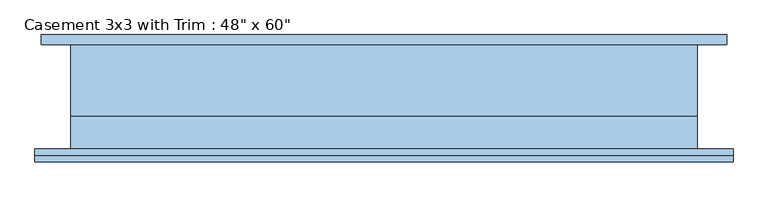
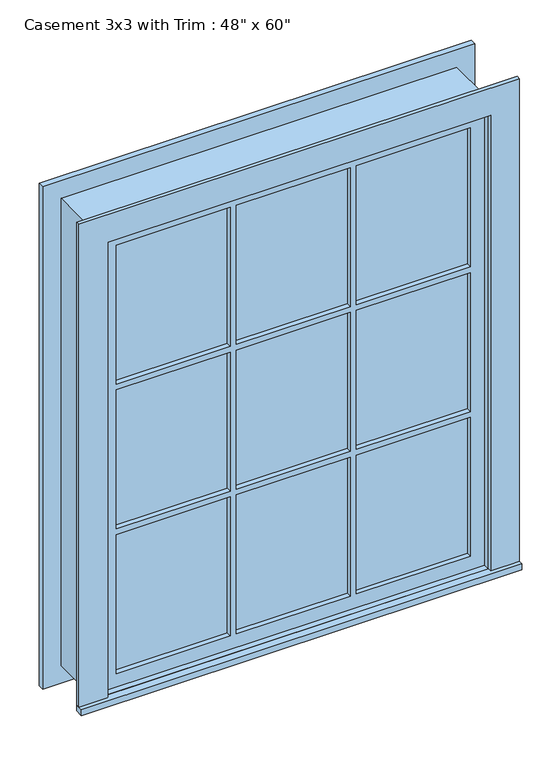
"""IFC4 building model written with IfcOpenShell, lengths in millimetres: window geometry."""

from ifc_helpers import new_model, si_unit, frame, origin, place, context, project, spatial, polyline, outline, extrude, source, transform, mapped, element, save


def window_4f803b43(model_context):
    return source(origin(), model_context, "Body", "SweptSolid", [
        extrude(outline(polyline([(-679.45, -127.0), (-679.45, -101.6), (679.45, -101.6), (679.45, -127.0), (-679.45, -127.0)])), frame((0.0, 0.0, 609.6), z_axis=(0.0, 0.0, 1.0), x_axis=(1.0, 0.0, 0.0)), (0.0, 0.0, 1.0), 19.05),
        extrude(outline(polyline([(2114.55, -590.55), (2114.55, 590.55), (628.65, 590.55), (628.65, 679.45), (2203.45, 679.45), (2203.45, -679.45), (628.65, -679.45), (628.65, -590.55), (2114.55, -590.55)])), frame((0.0, -114.3, 0.0), z_axis=(0.0, 1.0, 0.0), x_axis=(0.0, 0.0, 1.0)), (0.0, 0.0, 1.0), 12.7),
        extrude(outline(polyline([(194.7333333, -66.675), (194.7333333, -53.975), (546.1, -53.975), (546.1, -66.675), (194.7333333, -66.675)])), frame((0.0, 0.0, 1617.1333333), z_axis=(0.0, 0.0, 1.0), x_axis=(1.0, 0.0, 0.0)), (0.0, 0.0, 1.0), 452.9666667),
        extrude(outline(polyline([(-175.6833333, -66.675), (-175.6833333, -53.975), (175.6833333, -53.975), (175.6833333, -66.675), (-175.6833333, -66.675)])), frame((0.0, 0.0, 1617.1333333), z_axis=(0.0, 0.0, 1.0), x_axis=(1.0, 0.0, 0.0)), (0.0, 0.0, 1.0), 452.9666667),
        extrude(outline(polyline([(-546.1, -66.675), (-546.1, -53.975), (-194.7333333, -53.975), (-194.7333333, -66.675), (-546.1, -66.675)])), frame((0.0, 0.0, 1617.1333333), z_axis=(0.0, 0.0, 1.0), x_axis=(1.0, 0.0, 0.0)), (0.0, 0.0, 1.0), 452.9666667),
        extrude(outline(polyline([(-546.1, -66.675), (-546.1, -53.975), (-194.7333333, -53.975), (-194.7333333, -66.675), (-546.1, -66.675)])), frame((0.0, 0.0, 1145.1166667), z_axis=(0.0, 0.0, 1.0), x_axis=(1.0, 0.0, 0.0)), (0.0, 0.0, 1.0), 452.9666667),
        extrude(outline(polyline([(-175.6833333, -66.675), (-175.6833333, -53.975), (175.6833333, -53.975), (175.6833333, -66.675), (-175.6833333, -66.675)])), frame((0.0, 0.0, 1145.1166667), z_axis=(0.0, 0.0, 1.0), x_axis=(1.0, 0.0, 0.0)), (0.0, 0.0, 1.0), 452.9666667),
        extrude(outline(polyline([(194.7333333, -66.675), (194.7333333, -53.975), (546.1, -53.975), (546.1, -66.675), (194.7333333, -66.675)])), frame((0.0, 0.0, 1145.1166667), z_axis=(0.0, 0.0, 1.0), x_axis=(1.0, 0.0, 0.0)), (0.0, 0.0, 1.0), 452.9666667),
        extrude(outline(polyline([(194.7333333, -66.675), (194.7333333, -53.975), (546.1, -53.975), (546.1, -66.675), (194.7333333, -66.675)])), frame((0.0, 0.0, 673.1), z_axis=(0.0, 0.0, 1.0), x_axis=(1.0, 0.0, 0.0)), (0.0, 0.0, 1.0), 452.9666667),
        extrude(outline(polyline([(-175.6833333, -66.675), (-175.6833333, -53.975), (175.6833333, -53.975), (175.6833333, -66.675), (-175.6833333, -66.675)])), frame((0.0, 0.0, 673.1), z_axis=(0.0, 0.0, 1.0), x_axis=(1.0, 0.0, 0.0)), (0.0, 0.0, 1.0), 452.9666667),
        extrude(outline(polyline([(-546.1, -66.675), (-546.1, -53.975), (-194.7333333, -53.975), (-194.7333333, -66.675), (-546.1, -66.675)])), frame((0.0, 0.0, 673.1), z_axis=(0.0, 0.0, 1.0), x_axis=(1.0, 0.0, 0.0)), (0.0, 0.0, 1.0), 452.9666667),
        extrude(outline(polyline([(2190.75, 666.75), (2190.75, -666.75), (552.45, -666.75), (552.45, 666.75), (2190.75, 666.75)]), holes=[polyline([(2101.85, 577.85), (641.35, 577.85), (641.35, -577.85), (2101.85, -577.85), (2101.85, 577.85)])]), frame((0.0, 101.6, 0.0), z_axis=(0.0, 1.0, 0.0), x_axis=(0.0, 0.0, 1.0)), (0.0, 0.0, 1.0), 19.05),
        extrude(outline(polyline([(2114.55, -590.55), (628.65, -590.55), (628.65, 590.55), (2114.55, 590.55), (2114.55, -590.55)]), holes=[polyline([(2070.1, -194.7333333), (1617.1333333, -194.7333333), (1617.1333333, -546.1), (2070.1, -546.1), (2070.1, -194.7333333)]), polyline([(1598.0833333, -194.7333333), (1145.1166667, -194.7333333), (1145.1166667, -546.1), (1598.0833333, -546.1), (1598.0833333, -194.7333333)]), polyline([(1126.0666667, -194.7333333), (673.1, -194.7333333), (673.1, -546.1), (1126.0666667, -546.1), (1126.0666667, -194.7333333)]), polyline([(2070.1, 175.6833333), (1617.1333333, 175.6833333), (1617.1333333, -175.6833333), (2070.1, -175.6833333), (2070.1, 175.6833333)]), polyline([(1598.0833333, 175.6833333), (1145.1166667, 175.6833333), (1145.1166667, -175.6833333), (1598.0833333, -175.6833333), (1598.0833333, 175.6833333)]), polyline([(1126.0666667, 175.6833333), (673.1, 175.6833333), (673.1, -175.6833333), (1126.0666667, -175.6833333), (1126.0666667, 175.6833333)]), polyline([(2070.1, 546.1), (1617.1333333, 546.1), (1617.1333333, 194.7333333), (2070.1, 194.7333333), (2070.1, 546.1)]), polyline([(1598.0833333, 546.1), (1145.1166667, 546.1), (1145.1166667, 194.7333333), (1598.0833333, 194.7333333), (1598.0833333, 546.1)]), polyline([(1126.0666667, 546.1), (673.1, 546.1), (673.1, 194.7333333), (1126.0666667, 194.7333333), (1126.0666667, 546.1)])]), frame((0.0, -82.55, 0.0), z_axis=(0.0, 1.0, 0.0), x_axis=(0.0, 0.0, 1.0)), (0.0, 0.0, 1.0), 44.45),
        extrude(outline(polyline([(2133.6, -609.6), (609.6, -609.6), (609.6, 609.6), (2133.6, 609.6), (2133.6, -609.6)]), holes=[polyline([(2101.85, -577.85), (2101.85, 577.85), (641.35, 577.85), (641.35, -577.85), (2101.85, -577.85)])]), frame((0.0, -38.1, 0.0), z_axis=(0.0, 1.0, 0.0), x_axis=(0.0, 0.0, 1.0)), (0.0, 0.0, 1.0), 139.7),
        extrude(outline(polyline([(2133.6, 609.6), (2133.6, -609.6), (609.6, -609.6), (609.6, 609.6), (2133.6, 609.6)]), holes=[polyline([(2114.55, 590.55), (628.65, 590.55), (628.65, -590.55), (2114.55, -590.55), (2114.55, 590.55)])]), frame((0.0, -101.6, 0.0), z_axis=(0.0, 1.0, 0.0), x_axis=(0.0, 0.0, 1.0)), (0.0, 0.0, 1.0), 63.5),
    ])


if __name__ == "__main__":
    model = new_model("IFC4")
    model_context = context("Model", 3, world=origin())
    ifc_project = project(units=[si_unit("LENGTHUNIT", "METRE", prefix="MILLI")], contexts=[model_context])
    site = spatial("IfcSite", under=ifc_project)
    building = spatial("IfcBuilding", under=site)
    placement = place(None, origin())
    window_shape = window_4f803b43(model_context)
    element("IfcWindow", 1, ObjectType="Casement 3x3 with Trim : 48\" x 60\"", at=placement, inside=building, context=model_context, shape_type="MappedRepresentation", body=[
        mapped(window_shape, transform((0.0, 0.0, 0.0), x_axis=(1.0, 0.0, 0.0), y_axis=(0.0, 1.0, 0.0), z_axis=(0.0, 0.0, 1.0))),
    ])
    save(model, "model.ifc")

# Revit data of these elements
# Type "Casement 3x3 with Trim : 48\" x 60\""
#   Type Mark = "11"
#   Construction Type Id = "GSP4R"
#   Assembly Code = "B2020100"
#   Analytic Construction = "1/8 in Pilkington single glazing"
#   Visual Light Transmittance = 0.9
#   Solar Heat Gain Coefficient = 0.78
#   Heat Transfer Coefficient (U) = 0.6496 BTU/(h·ft²·°F)
#   Height = 5' - 0"
#   Default Sill Height = 2' - 0"
#   Trim Projection - Ext. = 0' - 0 1/2"
#   Trim Projection - Int. = 0' - 0 3/4"
#   Trim Width - Exterior = 0' - 3 1/2"
#   Trim Width - Interior = 0' - 3 1/2"
#   Width = 4' - 0"
#   Window Inset = 0' - 0 3/4"
#   Define Thermal Properties by = 1
#   Glass Pane Material = Glass
#   Sash Material = Sash
#   Trim Exterior Material = Trim
#   Trim Interior Material = Trim
#   Wall Closure = (empty or 0)
# Element 1 (IfcWindow, "Casement 3x3 with Trim : 48\" x 60\"")
#   Materials on its faces: "Sash", "Glass", "Trim"
# Materials
#   "Glass": class "Glass", colour RGB 0 128 192, transparency 0.75, Description = "Soda Lime Glass", Cost = 0
#   "Sash": class "Wood", colour RGB 224 178 126, transparency 0
#   "Trim": class "Wood", colour RGB 224 178 126, transparency 0
